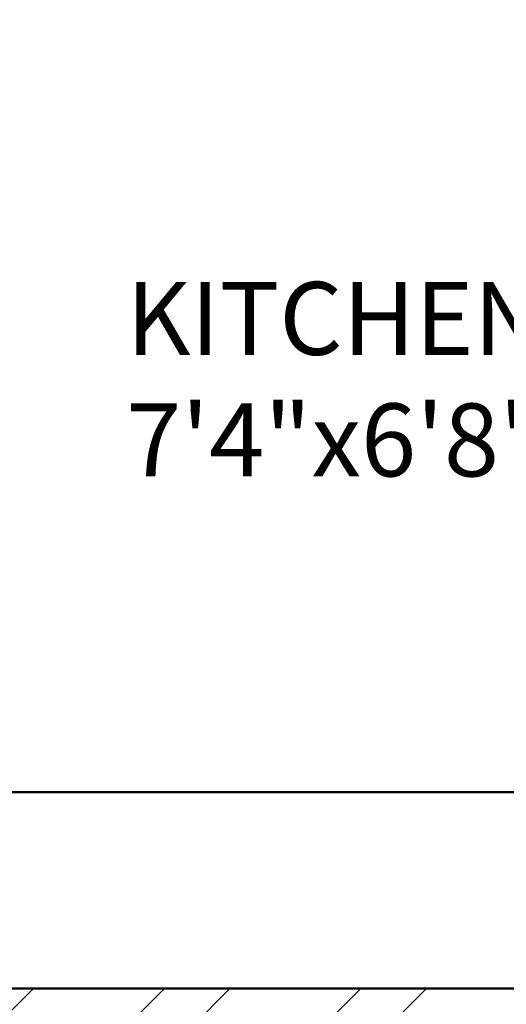
# Model space of a CAD drawing. Units: inches. Extents: x 1901 to 2863, y 888 to 2433.
# Tile 6 of 91: x 2053 to 2086, y 1442 to 1510. Entities that reach past the tile are written whole.
import ezdxf

# ---------------------------------------------------------------- set-up
doc = ezdxf.new("R2010")
doc.units = ezdxf.units.IN
for name, color, linetype, lineweight in [('A-AREA-IDEN', 7, 'Continuous', 18), ('A-WALL', 7, 'Continuous', 50), ('A-WALL-PATT', 8, 'Continuous', 13)]:
    doc.layers.add(name, color=color, linetype=linetype, lineweight=lineweight)
doc.styles.get("Standard").update_dxf_attribs({"font": 'arial.ttf'})

msp = doc.modelspace()

# ---------------------------------------------------------------- hatches: boundary and pattern name
at = {"layer": 'A-WALL-PATT'}
h = msp.add_hatch(dxfattribs=at)
h.set_pattern_fill('ANSI32', color=256)
h.paths.add_polyline_path([(2192.501, 2274.134), (2141.264, 2274.134), (2141.264, 2269.634), (2192.501, 2269.634)])
h.paths.add_polyline_path([(2259.926, 2274.134), (2216.501, 2274.134), (2216.501, 2269.634), (2255.426, 2269.634), (2255.426, 2214.634), (2250.809, 2214.634), (2250.809, 2210.134), (2259.926, 2210.134), (2259.926, 2215.134), (2271.756, 2215.134), (2271.756, 2217.384), (2271.756, 2219.634), (2259.926, 2219.634)])
h.paths.add_polyline_path([(2171.426, 2269.634), (2166.926, 2269.634), (2166.926, 2219.634), (2121.238, 2219.634), (2121.238, 2215.134), (2166.926, 2215.134), (2166.926, 2083.134), (2161.807, 2083.134), (2161.807, 2078.634), (2171.426, 2078.634), (2176.996, 2078.634), (2176.996, 2080.884), (2176.996, 2083.134), (2171.426, 2083.134), (2171.426, 2210.134), (2230.912, 2210.134), (2230.912, 2212.384), (2230.912, 2214.634), (2171.426, 2214.634)])
h.paths.add_polyline_path([(2117.264, 2274.134), (2089.426, 2274.134), (2089.426, 2219.634), (2081.136, 2219.634), (2081.136, 2215.134), (2089.426, 2215.134), (2098.004, 2215.134), (2098.004, 2217.384), (2098.004, 2219.634), (2093.926, 2219.634), (2093.926, 2269.634), (2117.264, 2269.634), (2117.264, 2271.884)])
h.paths.add_polyline_path([(2343.426, 2219.634), (2329.295, 2219.634), (2329.295, 2215.134), (2338.926, 2215.134), (2338.926, 2184.739), (2343.426, 2184.739)])
h.paths.add_polyline_path([(2338.926, 2083.134), (2329.295, 2083.134), (2208.966, 2083.134), (2208.966, 2078.634), (2338.926, 2078.634)])
h.paths.add_polyline_path([(2343.426, 2136.739), (2338.926, 2136.739), (2338.926, 1872.634), (2343.426, 1872.634)])
h.paths.add_polyline_path([(2343.426, 1863.634), (2397.68, 1863.634), (2397.68, 1821.634), (2384.138, 1821.634), (2384.138, 1812.634), (2418.33, 1812.634), (2418.33, 1817.134), (2418.33, 1821.634), (2406.68, 1821.634), (2406.68, 1863.634), (2459.499, 1863.634), (2459.499, 1821.634), (2447.138, 1821.634), (2447.138, 1812.634), (2459.499, 1812.634), (2468.499, 1812.634), (2468.499, 1872.634), (2394.426, 1872.634), (2334.426, 1872.634), (2334.426, 1812.634), (2343.426, 1812.634), (2353.251, 1812.634), (2353.251, 1821.634), (2343.426, 1821.634)])
h.paths.add_polyline_path([(2510.014, 1872.634), (2468.499, 1872.634), (2468.499, 1868.134), (2510.014, 1868.134)])
h.paths.add_polyline_path([(2514.009, 1817.134), (2468.499, 1817.134), (2468.499, 1812.634), (2482.114, 1812.634), (2482.114, 1800.606), (2486.614, 1800.606), (2486.614, 1812.634), (2514.009, 1812.634)])
h.paths.add_polyline_path([(2299.247, 1814.884), (2299.247, 1817.134), (2295.926, 1817.134), (2295.926, 1854.169), (2293.676, 1854.169), (2291.426, 1854.169), (2291.426, 1817.134), (2266.109, 1817.134), (2266.109, 1812.634), (2299.247, 1812.634)])
h.paths.add_polyline_path([(2218.109, 1817.134), (2206.46, 1817.134), (2171.426, 1817.134), (2171.426, 1949.134), (2190.1, 1949.134), (2190.1, 1953.634), (2163.468, 1953.634), (2163.468, 1949.134), (2166.926, 1949.134), (2166.926, 1817.134), (2114.297, 1817.134), (2114.297, 1812.634), (2218.109, 1812.634)])
h.paths.add_polyline_path([(2029.426, 1970.922), (2024.926, 1970.922), (2024.926, 1912.717), (2029.426, 1912.717)])
h.paths.add_polyline_path([(2132.297, 1953.634), (2113.926, 1953.634), (2113.926, 1975.888), (2111.676, 1975.888), (2109.426, 1975.888), (2109.426, 1953.634), (2029.426, 1953.634), (2029.426, 1949.134), (2132.297, 1949.134)])
h.paths.add_polyline_path([(2029.426, 1853.606), (2029.31, 1853.606), (2029.31, 1853.606), (2029.426, 1853.606), (2029.426, 1864.717), (2024.926, 1864.717), (2024.926, 1812.634), (2066.297, 1812.634), (2066.297, 1814.884), (2066.297, 1817.134), (2029.426, 1817.134)])
h.paths.add_polyline_path([(2122.926, 2010.088), (2120.676, 2010.088), (2118.426, 2010.088), (2118.426, 2006.134), (2029.426, 2006.134), (2029.426, 2001.634), (2109.426, 2001.634), (2109.426, 1998.041), (2113.926, 1998.041), (2113.926, 2001.634), (2122.926, 2001.634)])
h.paths.add_polyline_path([(2029.426, 2031.376), (2024.926, 2031.376), (2024.926, 1994.922), (2027.176, 1994.922), (2029.426, 1994.922)])
h.paths.add_polyline_path([(2029.426, 2136.739), (2024.926, 2136.739), (2024.926, 2067.376), (2027.176, 2067.376), (2029.426, 2067.376)])
h.paths.add_polyline_path([(2125.618, 2083.134), (2029.426, 2083.134), (2029.426, 2078.634), (2118.426, 2078.634), (2118.426, 2030.715), (2122.926, 2030.715), (2122.926, 2078.634), (2125.618, 2078.634)])
h.paths.add_polyline_path([(2029.426, 2215.134), (2040.468, 2215.134), (2040.468, 2217.384), (2040.468, 2219.634), (2024.926, 2219.634), (2024.926, 2184.739), (2029.426, 2184.739), (2029.426, 2187.778)])
h.paths.add_polyline_path([(2686.426, 2274.134), (2659.284, 2274.134), (2659.284, 2269.634), (2681.926, 2269.634), (2681.926, 2219.634), (2676.816, 2219.634), (2676.816, 2215.134), (2681.926, 2215.134), (2697.011, 2215.134), (2697.011, 2217.384), (2697.011, 2219.634), (2686.426, 2219.634)])
h.paths.add_polyline_path([(2609.926, 2269.634), (2635.284, 2269.634), (2635.284, 2274.134), (2571.431, 2274.134), (2571.431, 2269.634), (2605.426, 2269.634), (2605.426, 2214.634), (2549.098, 2214.634), (2549.098, 2210.134), (2605.426, 2210.134), (2605.426, 2083.134), (2601.014, 2083.134), (2601.014, 2080.884), (2601.014, 2078.634), (2609.926, 2078.634), (2616.162, 2078.634), (2616.162, 2080.884), (2616.162, 2083.134), (2609.926, 2083.134), (2609.926, 2215.134), (2651.465, 2215.134), (2651.465, 2217.384), (2651.465, 2219.634), (2609.926, 2219.634)])
h.paths.add_polyline_path([(2521.426, 2269.634), (2547.431, 2269.634), (2547.431, 2271.884), (2547.431, 2274.134), (2516.926, 2274.134), (2516.926, 2219.634), (2506.41, 2219.634), (2506.41, 2215.134), (2516.926, 2215.134), (2516.926, 2210.134), (2525.402, 2210.134), (2525.402, 2212.384), (2525.402, 2214.634), (2521.426, 2214.634)])
h.paths.add_polyline_path([(2456.011, 2219.634), (2439.426, 2219.634), (2439.426, 2187.888), (2443.926, 2187.888), (2443.926, 2215.134), (2456.011, 2215.134)])
h.paths.add_polyline_path([(2752.926, 2219.634), (2739.485, 2219.634), (2739.485, 2215.134), (2748.426, 2215.134), (2748.426, 2187.888), (2752.926, 2187.888)])
h.paths.add_polyline_path([(2752.926, 2139.888), (2748.426, 2139.888), (2748.426, 2083.134), (2648.416, 2083.134), (2648.416, 2078.634), (2654.926, 2078.634), (2654.926, 2039.437), (2659.426, 2039.437), (2659.426, 2078.634), (2748.426, 2078.634), (2748.426, 2063.429), (2752.926, 2063.429)])
h.paths.add_polyline_path([(2752.926, 2010.634), (2659.426, 2010.634), (2659.426, 2015.652), (2654.926, 2015.652), (2654.926, 2010.634), (2605.426, 2010.634), (2605.426, 1920.967), (2609.926, 1920.967), (2609.926, 2006.134), (2748.426, 2006.134), (2748.426, 1982.466), (2752.926, 1982.466)])
h.paths.add_polyline_path([(2752.926, 2027.429), (2748.426, 2027.429), (2748.426, 2010.634), (2752.926, 2010.634)])
h.paths.add_polyline_path([(2748.426, 1886.134), (2609.926, 1886.134), (2609.926, 1889.719), (2605.426, 1889.719), (2605.426, 1861.262), (2609.926, 1861.262), (2609.926, 1881.634), (2748.426, 1881.634)])
h.paths.add_polyline_path([(2456.855, 2228.831), (2498.401, 2228.831), (2498.401, 2247.488), (2456.855, 2247.488)], flags=9)
h.paths.add_polyline_path([(2038.602, 2237.418), (2080.174, 2237.418), (2080.174, 2256.075), (2038.602, 2256.075)], flags=9)
h.paths.add_polyline_path([(2292.009, 1062.394), (2539.932, 1062.394), (2539.932, 1099.487), (2292.009, 1099.487)], flags=9)
h.paths.add_polyline_path([(2424.91, 1832.253), (2448.513, 1832.253), (2448.513, 1846.678), (2424.91, 1846.678)], flags=25)
h.paths.add_polyline_path([(2359.076, 1832.253), (2382.678, 1832.253), (2382.678, 1846.678), (2359.076, 1846.678)], flags=25)
h.paths.add_polyline_path([(2352.899, 1684.802), (2367.543, 1684.802), (2367.543, 1697.167), (2352.899, 1697.167)], flags=9)
h.paths.add_polyline_path([(2079.288, 1755.826), (2169.024, 1755.826), (2169.024, 1774.372), (2079.288, 1774.372)], flags=9)
h.paths.add_polyline_path([(2404.09, 1373.857), (2404.09, 1463.593), (2385.544, 1463.593), (2385.544, 1373.857)], flags=9)
h.paths.add_polyline_path([(2268.091, 2236.371), (2309.636, 2236.371), (2309.636, 2255.028), (2268.091, 2255.028)], flags=9)
h.paths.add_polyline_path([(2575.96, 1700.951), (2665.696, 1700.951), (2665.696, 1719.498), (2575.96, 1719.498)], flags=9)
h.paths.add_polyline_path([(2302.962, 1878.474), (2329.524, 1878.474), (2329.524, 1888.777), (2302.962, 1888.777)], flags=9)
h.paths.add_polyline_path([(2097.415, 2240.576), (2126.573, 2240.576), (2126.573, 2259.233), (2097.415, 2259.233)], flags=9)
h.paths.add_polyline_path([(2208.725, 2246.124), (2237.882, 2246.124), (2237.882, 2264.781), (2208.725, 2264.781)], flags=9)
h.paths.add_polyline_path([(2038.147, 1925.958), (2076.987, 1925.958), (2076.987, 1944.615), (2038.147, 1944.615)], flags=9)
h.paths.add_polyline_path([(2239.144, 1926.672), (2288.465, 1926.672), (2288.465, 1945.329), (2239.144, 1945.329)], flags=9)
h.paths.add_polyline_path([(2175.429, 2007.33), (2212.356, 2007.33), (2212.356, 2025.987), (2175.429, 2025.987)], flags=9)
h.paths.add_polyline_path([(2225.034, 2091.794), (2263.875, 2091.794), (2263.875, 2110.451), (2225.034, 2110.451)], flags=9)
h.paths.add_polyline_path([(2035.398, 2098.478), (2074.238, 2098.478), (2074.238, 2117.135), (2035.398, 2117.135)], flags=9)
h.paths.add_polyline_path([(2050.102, 2029.209), (2083.26, 2029.209), (2083.26, 2047.866), (2050.102, 2047.866)], flags=9)
h.paths.add_polyline_path([(2069.677, 1956.719), (2098.835, 1956.719), (2098.835, 1975.376), (2069.677, 1975.376)], flags=25)
h.paths.add_polyline_path([(2328.62, 1753.336), (2361.663, 1753.336), (2361.663, 1771.993), (2328.62, 1771.993)], flags=9)
h.paths.add_polyline_path([(2395.162, 2060.888), (2395.162, 2140.654), (2378.676, 2140.654), (2378.676, 2060.888)], flags=9)
h.paths.add_polyline_path([(2463.728, 2059.02), (2492.886, 2059.02), (2492.886, 2077.677), (2463.728, 2077.677)], flags=9)
h.paths.add_polyline_path([(2458.027, 2181.536), (2496.868, 2181.536), (2496.868, 2200.194), (2458.027, 2200.194)], flags=9)
h.paths.add_polyline_path([(2527.577, 2243.074), (2556.735, 2243.074), (2556.735, 2261.731), (2527.577, 2261.731)], flags=9)
h.paths.add_polyline_path([(2694.461, 2232.767), (2736.033, 2232.767), (2736.033, 2251.425), (2694.461, 2251.425)], flags=9)
h.paths.add_polyline_path([(2637.821, 2249.225), (2666.979, 2249.225), (2666.979, 2267.882), (2637.821, 2267.882)], flags=9)
h.paths.add_polyline_path([(2623.687, 2183.541), (2662.528, 2183.541), (2662.528, 2202.199), (2623.687, 2202.199)], flags=9)
h.paths.add_polyline_path([(2691.965, 2021.5), (2725.124, 2021.5), (2725.124, 2040.157), (2691.965, 2040.157)], flags=9)
h.paths.add_polyline_path([(2621.043, 1975.912), (2662.335, 1975.912), (2662.335, 1994.569), (2621.043, 1994.569)], flags=25)
h.paths.add_polyline_path([(2479.032, 1927.62), (2519.844, 1927.62), (2519.844, 1946.277), (2479.032, 1946.277)], flags=9)
h.paths.add_polyline_path([(2670.941, 1849.076), (2716.005, 1849.076), (2716.005, 1867.734), (2670.941, 1867.734)], flags=9)
h.paths.add_polyline_path([(2523.613, 1782.956), (2550.175, 1782.956), (2550.175, 1793.26), (2523.613, 1793.26)], flags=9)
h.paths.add_polyline_path([(2450.841, 1207.331), (2492.386, 1207.331), (2492.386, 1225.989), (2450.841, 1225.989)], flags=9)
h.paths.add_polyline_path([(2527.751, 1203.841), (2556.908, 1203.841), (2556.908, 1222.499), (2527.751, 1222.499)], flags=9)
h.paths.add_polyline_path([(2639.111, 1207.2), (2668.268, 1207.2), (2668.268, 1225.857), (2639.111, 1225.857)], flags=9)
h.paths.add_polyline_path([(2692.594, 1218.965), (2734.167, 1218.965), (2734.167, 1237.623), (2692.594, 1237.623)], flags=9)
h.paths.add_polyline_path([(2669.266, 1366.329), (2708.106, 1366.329), (2708.106, 1384.987), (2669.266, 1384.987)], flags=9)
h.paths.add_polyline_path([(2463.313, 1358.031), (2502.153, 1358.031), (2502.153, 1376.688), (2463.313, 1376.688)], flags=9)
h.paths.add_polyline_path([(2494.725, 1449.963), (2531.652, 1449.963), (2531.652, 1468.62), (2494.725, 1468.62)], flags=9)
h.paths.add_polyline_path([(2675.565, 1422.157), (2708.724, 1422.157), (2708.724, 1440.815), (2675.565, 1440.815)], flags=9)
h.paths.add_polyline_path([(2685.634, 1493.891), (2714.792, 1493.891), (2714.792, 1512.548), (2685.634, 1512.548)], flags=9)
h.paths.add_polyline_path([(2686.805, 1529.913), (2725.645, 1529.913), (2725.645, 1548.57), (2686.805, 1548.57)], flags=9)
h.paths.add_polyline_path([(2503.651, 1537.991), (2552.972, 1537.991), (2552.972, 1556.648), (2503.651, 1556.648)], flags=9)
h.paths.add_polyline_path([(2291.713, 1643.504), (2318.275, 1643.504), (2318.275, 1653.807), (2291.713, 1653.807)], flags=9)
h.paths.add_polyline_path([(2450.626, 1610.52), (2477.189, 1610.52), (2477.189, 1620.824), (2450.626, 1620.824)], flags=9)
h.paths.add_polyline_path([(2359.985, 1551.814), (2422.253, 1551.814), (2422.253, 1562.117), (2359.985, 1562.117)], flags=9)
h.paths.add_polyline_path([(2280.106, 1249.006), (2321.651, 1249.006), (2321.651, 1267.663), (2280.106, 1267.663)], flags=9)
h.paths.add_polyline_path([(2164.057, 1274.232), (2193.215, 1274.232), (2193.215, 1292.889), (2164.057, 1292.889)], flags=9)
h.paths.add_polyline_path([(2118.21, 1277.694), (2151.252, 1277.694), (2151.252, 1296.351), (2118.21, 1296.351)], flags=9)
h.paths.add_polyline_path([(2031.946, 1268.529), (2073.519, 1268.529), (2073.519, 1287.187), (2031.946, 1287.187)], flags=9)
h.paths.add_polyline_path([(2050.199, 1409.079), (2089.04, 1409.079), (2089.04, 1427.736), (2050.199, 1427.736)], flags=9)
h.paths.add_polyline_path([(2243.743, 1421.032), (2282.584, 1421.032), (2282.584, 1439.689), (2243.743, 1439.689)], flags=9)
h.paths.add_polyline_path([(2190.746, 1509.769), (2231.558, 1509.769), (2231.558, 1528.426), (2190.746, 1528.426)], flags=9)
h.paths.add_polyline_path([(2058.392, 1475.415), (2091.55, 1475.415), (2091.55, 1494.073), (2058.392, 1494.073)], flags=9)
h.paths.add_polyline_path([(2062.447, 1553.09), (2091.605, 1553.09), (2091.605, 1571.747), (2062.447, 1571.747)], flags=9)
h.paths.add_polyline_path([(2219.524, 1590.365), (2266.147, 1590.365), (2266.147, 1609.022), (2219.524, 1609.022)], flags=9)
h.paths.add_polyline_path([(2041.072, 1584.188), (2079.912, 1584.188), (2079.912, 1602.845), (2041.072, 1602.845)], flags=9)
h = msp.add_hatch(dxfattribs=at)
h.set_pattern_fill('ANSI32', color=256)
h.paths.add_polyline_path([(2443.926, 2139.888), (2439.426, 2139.888), (2439.426, 2069.348), (2441.676, 2069.348), (2443.926, 2069.348), (2443.926, 2078.634), (2521.926, 2078.634), (2521.926, 2075.067), (2524.176, 2075.067), (2526.426, 2075.067), (2526.426, 2078.634), (2571.755, 2078.634), (2571.755, 2080.884), (2571.755, 2083.134), (2443.926, 2083.134)])
h.paths.add_polyline_path([(2526.426, 2054.634), (2524.176, 2054.634), (2521.926, 2054.634), (2521.926, 2030.634), (2443.926, 2030.634), (2443.926, 2045.348), (2439.426, 2045.348), (2439.426, 1983.867), (2443.926, 1983.867), (2443.926, 2026.134), (2521.926, 2026.134), (2526.426, 2026.134)])
h.paths.add_polyline_path([(2443.926, 1923.867), (2439.426, 1923.867), (2439.426, 1872.634), (2443.926, 1872.634)])
h.paths.add_polyline_path([(2636.233, 1766.134), (2609.926, 1766.134), (2609.926, 1779.785), (2605.426, 1779.785), (2605.426, 1766.134), (2486.614, 1766.134), (2486.614, 1770.671), (2482.114, 1770.671), (2482.114, 1766.134), (2482.114, 1761.634), (2636.233, 1761.634), (2636.233, 1763.884)])
h.paths.add_polyline_path([(2519.536, 1663.384), (2519.536, 1665.634), (2494.926, 1665.634), (2481.831, 1665.634), (2481.831, 1663.384), (2481.831, 1661.134), (2490.426, 1661.134), (2490.426, 1640.157), (2494.926, 1640.157), (2494.926, 1661.134), (2519.536, 1661.134)])
h.paths.add_polyline_path([(2443.926, 1712.134), (2443.926, 1716.634), (2414.464, 1716.634), (2414.464, 1712.134), (2439.426, 1712.134), (2439.426, 1545.507), (2443.926, 1545.507), (2443.926, 1661.134), (2448.475, 1661.134), (2448.475, 1665.634), (2443.926, 1665.634)])
h.paths.add_polyline_path([(2343.426, 1712.134), (2365.525, 1712.134), (2365.525, 1714.384), (2365.525, 1716.634), (2333.871, 1716.634), (2333.871, 1714.384), (2333.871, 1712.134), (2338.926, 1712.134), (2338.926, 1575.634), (2338.926, 1545.507), (2343.426, 1545.507), (2343.426, 1547.507), (2343.426, 1580.134)])
h.paths.add_polyline_path([(2752.926, 1665.634), (2579.536, 1665.634), (2579.536, 1661.134), (2615.926, 1661.134), (2615.926, 1529.134), (2598.931, 1529.134), (2598.931, 1524.634), (2623.127, 1524.634), (2623.127, 1526.884), (2623.127, 1529.134), (2620.426, 1529.134), (2620.426, 1661.134), (2748.426, 1661.134), (2748.426, 1633.499), (2752.926, 1633.499)])
h.paths.add_polyline_path([(2752.926, 1419.929), (2748.426, 1419.929), (2748.426, 1400.134), (2659.426, 1400.134), (2659.426, 1444.333), (2657.176, 1444.333), (2654.926, 1444.333), (2654.926, 1400.134), (2643.649, 1400.134), (2643.649, 1395.634), (2748.426, 1395.634), (2748.426, 1364.035), (2752.926, 1364.035)])
h.paths.add_polyline_path([(2752.926, 1492.878), (2748.426, 1492.878), (2748.426, 1476.634), (2667.426, 1476.634), (2667.426, 1479.71), (2665.176, 1479.71), (2662.926, 1479.71), (2662.926, 1476.634), (2654.926, 1476.634), (2654.926, 1469.536), (2659.426, 1469.536), (2659.426, 1472.134), (2748.426, 1472.134), (2748.426, 1455.929), (2752.926, 1455.929)])
h.paths.add_polyline_path([(2752.926, 1304.035), (2748.426, 1304.035), (2748.426, 1263.634), (2738.66, 1263.634), (2738.66, 1259.134), (2752.926, 1259.134)])
h.paths.add_polyline_path([(2685.926, 1259.134), (2695.49, 1259.134), (2695.49, 1261.384), (2695.49, 1263.634), (2677.837, 1263.634), (2677.837, 1261.384), (2677.837, 1259.134), (2681.426, 1259.134), (2681.426, 1203.634), (2653.277, 1203.634), (2653.277, 1199.134), (2685.926, 1199.134), (2685.926, 1203.634)])
h.paths.add_polyline_path([(2609.426, 1395.634), (2611.848, 1395.634), (2611.848, 1400.134), (2598.888, 1400.134), (2598.888, 1397.884), (2598.888, 1395.634), (2604.926, 1395.634), (2604.926, 1268.134), (2554.726, 1268.134), (2554.726, 1265.884), (2554.726, 1263.634), (2604.926, 1263.634), (2604.926, 1203.634), (2571.306, 1203.634), (2571.306, 1199.134), (2604.926, 1199.134), (2629.277, 1199.134), (2629.277, 1201.384), (2629.277, 1203.634), (2609.426, 1203.634), (2609.426, 1258.634), (2609.426, 1259.134), (2654.804, 1259.134), (2654.804, 1263.634), (2609.426, 1263.634)])
h.paths.add_polyline_path([(2443.926, 1304.035), (2439.426, 1304.035), (2439.426, 1259.134), (2443.926, 1259.134), (2456.16, 1259.134), (2456.16, 1261.384), (2456.16, 1263.634), (2443.926, 1263.634)])
h.paths.add_polyline_path([(2525.426, 1263.634), (2531.778, 1263.634), (2531.778, 1268.134), (2520.926, 1268.134), (2520.926, 1263.634), (2511.409, 1263.634), (2511.409, 1259.134), (2520.926, 1259.134), (2520.926, 1199.134), (2547.306, 1199.134), (2547.306, 1201.384), (2547.306, 1203.634), (2525.426, 1203.634)])
h.paths.add_polyline_path([(2443.926, 1434.842), (2439.426, 1434.842), (2439.426, 1364.035), (2441.676, 1364.035), (2443.926, 1364.035)])
h.paths.add_polyline_path([(2567.134, 1400.134), (2443.926, 1400.134), (2443.926, 1395.634), (2567.134, 1395.634)])
h.paths.add_polyline_path([(2443.926, 1545.507), (2439.426, 1545.507), (2439.426, 1494.842), (2443.926, 1494.842)])
h.paths.add_polyline_path([(2494.926, 1553.349), (2492.676, 1553.349), (2490.426, 1553.349), (2490.426, 1524.634), (2494.926, 1524.634), (2525.936, 1524.634), (2525.936, 1526.884), (2525.936, 1529.134), (2494.926, 1529.134)])
h.paths.add_polyline_path([(2752.926, 1573.499), (2748.426, 1573.499), (2748.426, 1529.134), (2657.759, 1529.134), (2657.759, 1524.634), (2662.926, 1524.634), (2662.926, 1498.631), (2667.426, 1498.631), (2667.426, 1524.634), (2748.426, 1524.634), (2748.426, 1516.878), (2752.926, 1516.878)])
h.paths.add_polyline_path([(2038.602, 2237.418), (2080.174, 2237.418), (2080.174, 2256.075), (2038.602, 2256.075)], flags=9)
h.paths.add_polyline_path([(2292.009, 1062.394), (2539.932, 1062.394), (2539.932, 1099.487), (2292.009, 1099.487)], flags=9)
h.paths.add_polyline_path([(2424.91, 1832.253), (2448.513, 1832.253), (2448.513, 1846.678), (2424.91, 1846.678)], flags=9)
h.paths.add_polyline_path([(2359.076, 1832.253), (2382.678, 1832.253), (2382.678, 1846.678), (2359.076, 1846.678)], flags=9)
h.paths.add_polyline_path([(2352.899, 1684.802), (2367.543, 1684.802), (2367.543, 1697.167), (2352.899, 1697.167)], flags=9)
h.paths.add_polyline_path([(2079.288, 1755.826), (2169.024, 1755.826), (2169.024, 1774.372), (2079.288, 1774.372)], flags=9)
h.paths.add_polyline_path([(2404.09, 1373.857), (2404.09, 1463.593), (2385.544, 1463.593), (2385.544, 1373.857)], flags=9)
h.paths.add_polyline_path([(2268.091, 2236.371), (2309.636, 2236.371), (2309.636, 2255.028), (2268.091, 2255.028)], flags=9)
h.paths.add_polyline_path([(2575.96, 1700.951), (2665.696, 1700.951), (2665.696, 1719.498), (2575.96, 1719.498)], flags=9)
h.paths.add_polyline_path([(2302.962, 1878.474), (2329.524, 1878.474), (2329.524, 1888.777), (2302.962, 1888.777)], flags=9)
h.paths.add_polyline_path([(2097.415, 2240.576), (2126.573, 2240.576), (2126.573, 2259.233), (2097.415, 2259.233)], flags=9)
h.paths.add_polyline_path([(2208.725, 2246.124), (2237.882, 2246.124), (2237.882, 2264.781), (2208.725, 2264.781)], flags=9)
h.paths.add_polyline_path([(2038.147, 1925.958), (2076.987, 1925.958), (2076.987, 1944.615), (2038.147, 1944.615)], flags=9)
h.paths.add_polyline_path([(2239.144, 1926.672), (2288.465, 1926.672), (2288.465, 1945.329), (2239.144, 1945.329)], flags=9)
h.paths.add_polyline_path([(2175.429, 2007.33), (2212.356, 2007.33), (2212.356, 2025.987), (2175.429, 2025.987)], flags=9)
h.paths.add_polyline_path([(2225.034, 2091.794), (2263.875, 2091.794), (2263.875, 2110.451), (2225.034, 2110.451)], flags=9)
h.paths.add_polyline_path([(2035.398, 2098.478), (2074.238, 2098.478), (2074.238, 2117.135), (2035.398, 2117.135)], flags=9)
h.paths.add_polyline_path([(2050.102, 2029.209), (2083.26, 2029.209), (2083.26, 2047.866), (2050.102, 2047.866)], flags=9)
h.paths.add_polyline_path([(2069.677, 1956.719), (2098.835, 1956.719), (2098.835, 1975.376), (2069.677, 1975.376)], flags=9)
h.paths.add_polyline_path([(2328.62, 1753.336), (2361.663, 1753.336), (2361.663, 1771.993), (2328.62, 1771.993)], flags=9)
h.paths.add_polyline_path([(2395.162, 2060.888), (2395.162, 2140.654), (2378.676, 2140.654), (2378.676, 2060.888)], flags=9)
h.paths.add_polyline_path([(2463.728, 2059.02), (2492.886, 2059.02), (2492.886, 2077.677), (2463.728, 2077.677)], flags=9)
h.paths.add_polyline_path([(2458.027, 2181.536), (2496.868, 2181.536), (2496.868, 2200.194), (2458.027, 2200.194)], flags=9)
h.paths.add_polyline_path([(2456.855, 2228.831), (2498.401, 2228.831), (2498.401, 2247.488), (2456.855, 2247.488)], flags=9)
h.paths.add_polyline_path([(2527.577, 2243.074), (2556.735, 2243.074), (2556.735, 2261.731), (2527.577, 2261.731)], flags=9)
h.paths.add_polyline_path([(2694.461, 2232.767), (2736.033, 2232.767), (2736.033, 2251.425), (2694.461, 2251.425)], flags=9)
h.paths.add_polyline_path([(2637.821, 2249.225), (2666.979, 2249.225), (2666.979, 2267.882), (2637.821, 2267.882)], flags=9)
h.paths.add_polyline_path([(2623.687, 2183.541), (2662.528, 2183.541), (2662.528, 2202.199), (2623.687, 2202.199)], flags=9)
h.paths.add_polyline_path([(2691.965, 2021.5), (2725.124, 2021.5), (2725.124, 2040.157), (2691.965, 2040.157)], flags=9)
h.paths.add_polyline_path([(2621.043, 1975.912), (2662.335, 1975.912), (2662.335, 1994.569), (2621.043, 1994.569)], flags=9)
h.paths.add_polyline_path([(2479.032, 1927.62), (2519.844, 1927.62), (2519.844, 1946.277), (2479.032, 1946.277)], flags=9)
h.paths.add_polyline_path([(2670.941, 1849.076), (2716.005, 1849.076), (2716.005, 1867.734), (2670.941, 1867.734)], flags=9)
h.paths.add_polyline_path([(2523.613, 1782.956), (2550.175, 1782.956), (2550.175, 1793.26), (2523.613, 1793.26)], flags=9)
h.paths.add_polyline_path([(2450.841, 1207.331), (2492.386, 1207.331), (2492.386, 1225.989), (2450.841, 1225.989)], flags=9)
h.paths.add_polyline_path([(2527.751, 1203.841), (2556.908, 1203.841), (2556.908, 1222.499), (2527.751, 1222.499)], flags=9)
h.paths.add_polyline_path([(2639.111, 1207.2), (2668.268, 1207.2), (2668.268, 1225.857), (2639.111, 1225.857)], flags=9)
h.paths.add_polyline_path([(2692.594, 1218.965), (2734.167, 1218.965), (2734.167, 1237.623), (2692.594, 1237.623)], flags=9)
h.paths.add_polyline_path([(2669.266, 1366.329), (2708.106, 1366.329), (2708.106, 1384.987), (2669.266, 1384.987)], flags=25)
h.paths.add_polyline_path([(2463.313, 1358.031), (2502.153, 1358.031), (2502.153, 1376.688), (2463.313, 1376.688)], flags=9)
h.paths.add_polyline_path([(2494.725, 1449.963), (2531.652, 1449.963), (2531.652, 1468.62), (2494.725, 1468.62)], flags=9)
h.paths.add_polyline_path([(2675.565, 1422.157), (2708.724, 1422.157), (2708.724, 1440.815), (2675.565, 1440.815)], flags=25)
h.paths.add_polyline_path([(2685.634, 1493.891), (2714.792, 1493.891), (2714.792, 1512.548), (2685.634, 1512.548)], flags=9)
h.paths.add_polyline_path([(2686.805, 1529.913), (2725.645, 1529.913), (2725.645, 1548.57), (2686.805, 1548.57)], flags=25)
h.paths.add_polyline_path([(2503.651, 1537.991), (2552.972, 1537.991), (2552.972, 1556.648), (2503.651, 1556.648)], flags=9)
h.paths.add_polyline_path([(2291.713, 1643.504), (2318.275, 1643.504), (2318.275, 1653.807), (2291.713, 1653.807)], flags=9)
h.paths.add_polyline_path([(2450.626, 1610.52), (2477.189, 1610.52), (2477.189, 1620.824), (2450.626, 1620.824)], flags=9)
h.paths.add_polyline_path([(2359.985, 1551.814), (2422.253, 1551.814), (2422.253, 1562.117), (2359.985, 1562.117)], flags=9)
h.paths.add_polyline_path([(2280.106, 1249.006), (2321.651, 1249.006), (2321.651, 1267.663), (2280.106, 1267.663)], flags=9)
h.paths.add_polyline_path([(2164.057, 1274.232), (2193.215, 1274.232), (2193.215, 1292.889), (2164.057, 1292.889)], flags=9)
h.paths.add_polyline_path([(2118.21, 1277.694), (2151.252, 1277.694), (2151.252, 1296.351), (2118.21, 1296.351)], flags=9)
h.paths.add_polyline_path([(2031.946, 1268.529), (2073.519, 1268.529), (2073.519, 1287.187), (2031.946, 1287.187)], flags=9)
h.paths.add_polyline_path([(2050.199, 1409.079), (2089.04, 1409.079), (2089.04, 1427.736), (2050.199, 1427.736)], flags=9)
h.paths.add_polyline_path([(2243.743, 1421.032), (2282.584, 1421.032), (2282.584, 1439.689), (2243.743, 1439.689)], flags=9)
h.paths.add_polyline_path([(2190.746, 1509.769), (2231.558, 1509.769), (2231.558, 1528.426), (2190.746, 1528.426)], flags=9)
h.paths.add_polyline_path([(2058.392, 1475.415), (2091.55, 1475.415), (2091.55, 1494.073), (2058.392, 1494.073)], flags=9)
h.paths.add_polyline_path([(2062.447, 1553.09), (2091.605, 1553.09), (2091.605, 1571.747), (2062.447, 1571.747)], flags=9)
h.paths.add_polyline_path([(2219.524, 1590.365), (2266.147, 1590.365), (2266.147, 1609.022), (2219.524, 1609.022)], flags=9)
h.paths.add_polyline_path([(2041.072, 1584.188), (2079.912, 1584.188), (2079.912, 1602.845), (2041.072, 1602.845)], flags=9)
h = msp.add_hatch(dxfattribs=at)
h.set_pattern_fill('ANSI32', color=256)
h.paths.add_polyline_path([(2182.933, 1716.634), (2024.926, 1716.634), (2024.926, 1681.702), (2029.326, 1681.702), (2029.326, 1712.134), (2154.326, 1712.134), (2154.326, 1580.134), (2148.524, 1580.134), (2148.524, 1577.884), (2148.524, 1575.634), (2194.93, 1575.634), (2194.93, 1580.134), (2158.826, 1580.134), (2158.826, 1712.134), (2182.933, 1712.134)])
h.paths.add_polyline_path([(2301.069, 1716.634), (2242.933, 1716.634), (2242.933, 1712.134), (2283.826, 1712.134), (2283.826, 1685.535), (2288.326, 1685.535), (2288.326, 1712.134), (2301.069, 1712.134)])
h.paths.add_polyline_path([(2288.326, 1600.411), (2286.076, 1600.411), (2283.826, 1600.411), (2283.826, 1580.134), (2270.601, 1580.134), (2270.601, 1575.634), (2288.326, 1575.634)])
h.paths.add_polyline_path([(2295.926, 1953.634), (2271.447, 1953.634), (2271.447, 1949.134), (2291.426, 1949.134), (2291.426, 1941.244), (2295.926, 1941.244)])
h.paths.add_polyline_path([(2098.376, 1244.134), (2082.326, 1244.134), (2082.326, 1302.134), (2086.523, 1302.134), (2086.523, 1306.634), (2067.456, 1306.634), (2067.456, 1302.134), (2077.826, 1302.134), (2077.826, 1239.634), (2098.376, 1239.634), (2098.376, 1241.884)])
h.paths.add_polyline_path([(2217.308, 1306.634), (2158.826, 1306.634), (2158.826, 1451.634), (2162.716, 1451.634), (2162.716, 1453.884), (2162.716, 1456.134), (2154.326, 1456.134), (2154.326, 1443.134), (2151.91, 1443.134), (2151.91, 1438.634), (2154.326, 1438.634), (2154.326, 1306.634), (2109.307, 1306.634), (2109.307, 1304.384), (2109.307, 1302.134), (2154.326, 1302.134), (2154.326, 1244.134), (2122.376, 1244.134), (2122.376, 1239.634), (2154.326, 1239.634), (2154.326, 1223.634), (2163.326, 1223.634), (2181.008, 1223.634), (2181.008, 1225.884), (2181.008, 1228.134), (2163.326, 1228.134), (2163.326, 1258.222), (2158.826, 1258.222), (2158.826, 1302.134), (2217.308, 1302.134)])
h.paths.add_polyline_path([(2259.991, 1306.634), (2238.299, 1306.634), (2238.299, 1304.384), (2238.299, 1302.134), (2242.826, 1302.134), (2242.826, 1228.134), (2205.008, 1228.134), (2205.008, 1223.634), (2247.326, 1223.634), (2247.326, 1302.134), (2259.991, 1302.134), (2259.991, 1304.384)])
h.paths.add_polyline_path([(2343.426, 1361.697), (2338.926, 1361.697), (2338.926, 1306.634), (2322.38, 1306.634), (2322.38, 1302.134), (2343.426, 1302.134)])
h.paths.add_polyline_path([(2343.426, 1470.397), (2338.926, 1470.397), (2338.926, 1456.134), (2193.726, 1456.134), (2193.726, 1453.884), (2193.726, 1451.634), (2338.926, 1451.634), (2338.926, 1421.697), (2343.426, 1421.697)])
h.paths.add_polyline_path([(2343.426, 1545.507), (2338.926, 1545.507), (2338.926, 1530.397), (2343.426, 1530.397)])
h.paths.add_polyline_path([(2029.326, 1466.83), (2024.926, 1466.83), (2024.926, 1409.825), (2029.326, 1409.825)])
h.paths.add_polyline_path([(2122.843, 1440.884), (2122.843, 1443.134), (2121.826, 1443.134), (2121.826, 1498.183), (2119.576, 1498.183), (2117.326, 1498.183), (2117.326, 1443.134), (2029.326, 1443.134), (2029.326, 1438.634), (2122.843, 1438.634)])
h.paths.add_polyline_path([(2029.326, 1543.053), (2024.926, 1543.053), (2024.926, 1502.83), (2029.326, 1502.83)])
h.paths.add_polyline_path([(2029.326, 1621.702), (2024.926, 1621.702), (2024.926, 1567.053), (2027.126, 1567.053), (2029.326, 1567.053), (2029.326, 1575.634), (2109.326, 1575.634), (2109.326, 1554.715), (2113.826, 1554.715), (2113.826, 1575.634), (2115.805, 1575.634), (2115.805, 1577.884), (2115.805, 1580.134), (2029.326, 1580.134)])
h.paths.add_polyline_path([(2121.826, 1527.634), (2117.326, 1527.634), (2113.826, 1527.634), (2113.826, 1533.011), (2111.576, 1533.011), (2109.326, 1533.011), (2109.326, 1527.634), (2029.326, 1527.634), (2029.326, 1523.134), (2117.326, 1523.134), (2117.326, 1519.43), (2121.826, 1519.43)])
h.paths.add_polyline_path([(2029.326, 1349.825), (2024.926, 1349.825), (2024.926, 1302.134), (2036.277, 1302.134), (2036.277, 1306.634), (2029.326, 1306.634)])

# ---------------------------------------------------------------- linework, layer by layer
at = {"layer": 'A-WALL'}
for p, q in [((2117.326, 1456.597), (2043.059, 1456.597)), ((2117.326, 1443.134), (2029.326, 1443.134))]:
    msp.add_line(p, q, dxfattribs=at)

# ---------------------------------------------------------------- texts
at = {"layer": 'A-AREA-IDEN', "insert": (2060.154, 1491.585), "char_height": 5, "attachment_point": 1}
msp.add_mtext_dynamic_manual_height_columns('KITCHEN\\P7\'4"x6\'8"', width=173.05788, gutter_width=12.5, heights=[0], dxfattribs=at)

doc.saveas('drawing.dxf')
